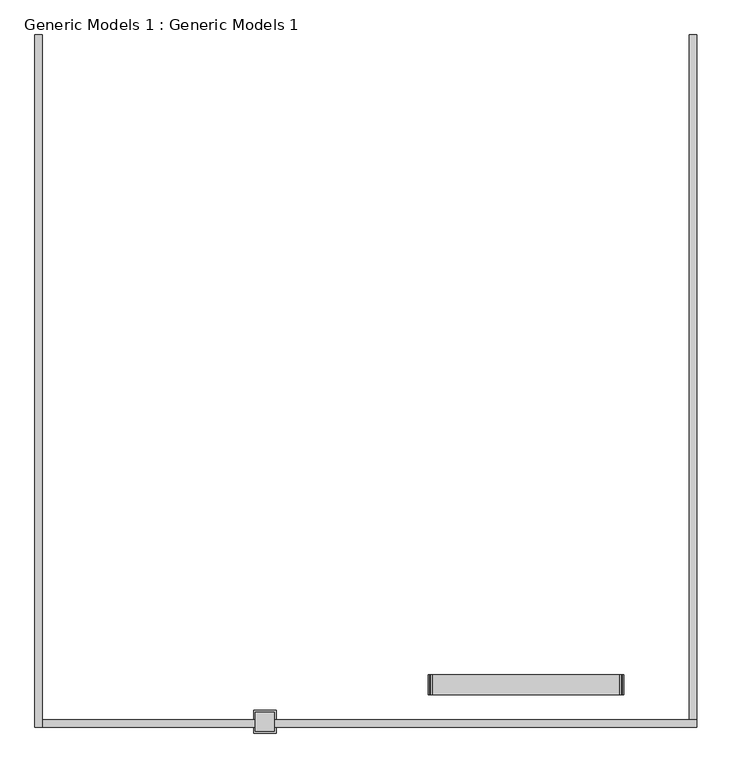
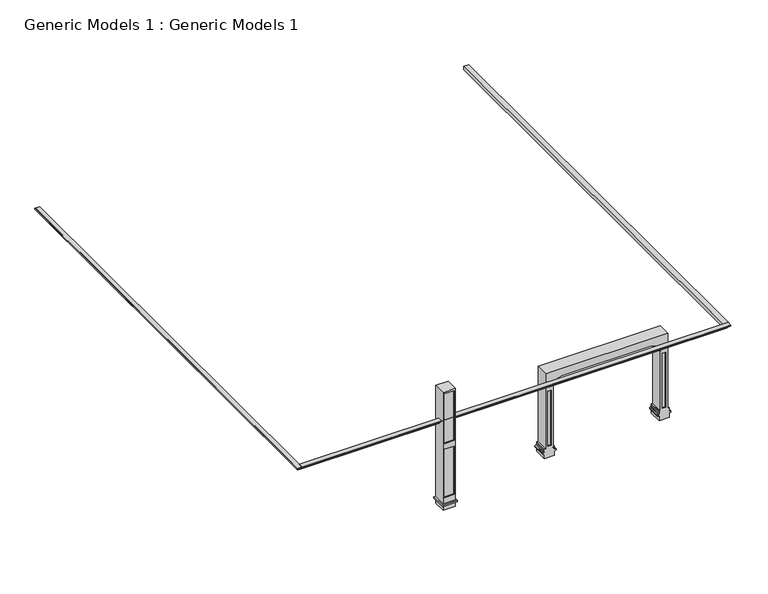
"""IFC4 building model written with IfcOpenShell, lengths in millimetres: proxy geometry, Generic Models 1 : Generic Models 1."""

from ifc_helpers import new_model, si_unit, point, frame, frame_2d, origin, origin_with_axes, place, context, project, spatial, polyline, circle_curve, ellipse_curve, trimmed, segment, composite_curve, outline, extrude, faceted_brep, source, transform, mapped, element, save
from ifc_brep_helpers import plane_surface, cylinder_surface, revolved_surface, advanced_brep


def generic_models_1_generic_models_1_5e55def3(model_context):
    return source(origin(), model_context, "Body", "SolidModel", [
        faceted_brep([(-2619.8591656, -8802.2949916, 5105.4), (-3127.8591656, -8802.2949916, 5105.4), (-3127.8591656, -9310.2949916, 5105.4), (-2619.8591656, -9310.2949916, 5105.4), (-2619.8591656, -8802.2949916, 279.4), (-2619.8591656, -9310.2949916, 279.4), (-3127.8591656, -9310.2949916, 279.4), (-3127.8591656, -8802.2949916, 279.4), (-2670.6591656, -9310.2949916, 532.3431413), (-3077.0591656, -9310.2949916, 532.3431413), (-3077.0591656, -9310.2949916, 2624.1375), (-2670.6591656, -9310.2949916, 2624.1375), (-2670.6591656, -9310.2949916, 5029.2), (-2670.6591656, -9310.2949916, 2870.2), (-3077.0591656, -9310.2949916, 2870.2), (-3077.0591656, -9310.2949916, 5029.2), (-2670.6591656, -9259.4949916, 532.3431413), (-2670.6591656, -9259.4949916, 2624.1375), (-3077.0591656, -9259.4949916, 2624.1375), (-3077.0591656, -9259.4949916, 532.3431413), (-2670.6591656, -9259.4949916, 5029.2), (-3077.0591656, -9259.4949916, 5029.2), (-3077.0591656, -9259.4949916, 2870.2), (-2670.6591656, -9259.4949916, 2870.2)], [[[0, 1, 2, 3]], [[4, 5, 6, 7]], [[1, 0, 4, 7]], [[2, 1, 7, 6]], [[3, 2, 6, 5], [8, 9, 10, 11], [12, 13, 14, 15]], [[0, 3, 5, 4]], [[16, 17, 18, 19]], [[20, 21, 22, 23]], [[16, 19, 9, 8]], [[19, 18, 10, 9]], [[18, 17, 11, 10]], [[17, 16, 8, 11]], [[20, 23, 13, 12]], [[23, 22, 14, 13]], [[22, 21, 15, 14]], [[21, 20, 12, 15]]]),
        extrude(outline(polyline([(-3178.6591656, -9361.0949916), (-3178.6591656, -8751.4949916), (-2569.0591656, -8751.4949916), (-2569.0591656, -9361.0949916), (-3178.6591656, -9361.0949916)])), frame((0.0, 0.0, 203.2), z_axis=(0.0, 0.0, 1.0), x_axis=(1.0, 0.0, 0.0)), (0.0, 0.0, 1.0), 76.2),
        extrude(outline(polyline([(-3127.8591656, -9310.2949916), (-3127.8591656, -8802.2949916), (-2619.8591656, -8802.2949916), (-2619.8591656, -9310.2949916), (-3127.8591656, -9310.2949916)])), origin_with_axes(), (0.0, 0.0, 1.0), 203.2),
        advanced_brep(
        [(-9051.9249265, 9396.8050084, 3810.0), (-8848.7249265, 9396.8050084, 3810.0), (-8848.7249265, 9396.8050084, 3657.6), (-8924.9249265, 9396.8050084, 3657.6), (-8924.9249265, 9396.8050084, 3668.8560823), (-8939.0688442, 9396.8050084, 3683.0), (-8950.3249265, 9396.8050084, 3683.0), (-8950.3249265, 9396.8050084, 3708.4), (-8975.7249265, 9396.8050084, 3733.8), (-9001.1249265, 9396.8050084, 3733.8), (-9001.1249265, 9396.8050084, 3761.8750168), (-9023.8499097, 9396.8050084, 3784.6), (-9026.5249265, 9396.8050084, 3784.6), (-9051.9249265, 9396.8050084, 3784.6), (-9051.9249265, -9180.6199748, 3784.6), (-9051.9249265, -9183.2949916, 3784.6), (-9051.9249265, -9208.6949916, 3784.6), (-9051.9249265, -9208.6949916, 3810.0), (-9026.5249265, -9180.6199748, 3784.6), (-9026.5249265, -9183.2949916, 3784.6), (-9026.5249265, -9208.6949916, 3784.6), (-9023.8499097, -9180.6199748, 3784.6), (-8848.7249265, -9180.6199748, 3784.6), (-8848.7249265, -9208.6949916, 3784.6), (-9001.1249265, -9157.8949916, 3761.8750168), (-9001.1249265, -9157.8949916, 3733.8), (-8975.7249265, -9132.4949916, 3733.8), (-8848.7249265, -9132.4949916, 3733.8), (-8848.7249265, -9157.8949916, 3733.8), (-8950.3249265, -9107.0949916, 3708.4), (-8950.3249265, -9107.0949916, 3683.0), (-8939.0688442, -9095.8389093, 3683.0), (-8848.7249265, -9095.8389093, 3683.0), (-8848.7249265, -9107.0949916, 3683.0), (-8924.9249265, -9081.6949916, 3668.8560823), (-8924.9249265, -9081.6949916, 3657.6), (-8848.7249265, -9081.6949916, 3657.6), (-8848.7249265, -9208.6949916, 3810.0), (-8848.7249265, -9157.8949916, 3761.8750168), (-8848.7249265, -9107.0949916, 3708.4), (-8848.7249265, -9081.6949916, 3668.8560823)],
        [
            (0, 1),
            (1, 2),
            (2, 3),
            (3, 4),
            (4, 5, circle_curve(frame((-8939.0688442, 9396.8050084, 3668.8560823), z_axis=(0.0, -1.0, 0.0), x_axis=(0.0, 0.0, 1.0)), 14.1439177)),
            (5, 6),
            (6, 7),
            (7, 8, circle_curve(frame((-8975.7249265, 9396.8050084, 3708.4), z_axis=(0.0, -1.0, 0.0), x_axis=(0.0, 0.0, 1.0)), 25.4)),
            (8, 9),
            (9, 10),
            (10, 11, circle_curve(frame((-9023.8499097, 9396.8050084, 3761.8750168), z_axis=(0.0, -1.0, 0.0), x_axis=(0.0, 0.0, 1.0)), 22.7249832)),
            (11, 12),
            (12, 13),
            (13, 0),
            (13, 14),
            (14, 15),
            (15, 16),
            (16, 17),
            (17, 0),
            (12, 18),
            (18, 19),
            (19, 20),
            (20, 16),
            (11, 21),
            (21, 22),
            (22, 23),
            (23, 20),
            (10, 24),
            (24, 21, ellipse_curve(frame((-9023.8499097, -9180.6199748, 3761.8750168), z_axis=(0.7071067811865451, -0.7071067811865498, 0.0), x_axis=(-0.7071067811865497, -0.7071067811865452, 0.0)), 32.1379795, 22.7249832)),
            (9, 25),
            (25, 24),
            (8, 26),
            (26, 27),
            (27, 28),
            (28, 25),
            (7, 29),
            (29, 26, ellipse_curve(frame((-8975.7249265, -9132.4949916, 3708.4), z_axis=(0.7071067811865451, -0.7071067811865498, 0.0), x_axis=(-0.7071067811865497, -0.7071067811865452, 0.0)), 35.9210245, 25.4)),
            (6, 30),
            (30, 29),
            (5, 31),
            (31, 32),
            (32, 33),
            (33, 30),
            (4, 34),
            (34, 31, ellipse_curve(frame((-8939.0688442, -9095.8389093, 3668.8560823), z_axis=(0.7071067811865451, -0.7071067811865498, 0.0), x_axis=(-0.7071067811865497, -0.7071067811865452, 0.0)), 20.0025203, 14.1439177)),
            (3, 35),
            (35, 34),
            (2, 36),
            (36, 35),
            (1, 37),
            (37, 23),
            (22, 38, circle_curve(frame((-8848.7249265, -9180.6199748, 3761.8750168), z_axis=(-1.0, 0.0, 0.0), x_axis=(0.0, 0.0, 1.0)), 22.7249832)),
            (38, 28),
            (27, 39, circle_curve(frame((-8848.7249265, -9132.4949916, 3708.4), z_axis=(-1.0, 0.0, 0.0), x_axis=(0.0, 0.0, 1.0)), 25.4)),
            (39, 33),
            (32, 40, circle_curve(frame((-8848.7249265, -9095.8389093, 3668.8560823), z_axis=(-1.0, 0.0, 0.0), x_axis=(0.0, 0.0, 1.0)), 14.1439177)),
            (40, 36),
            (17, 37),
            (40, 34),
            (24, 38),
            (29, 39),
        ],
        [
            plane_surface(frame((-8848.7249265, 9396.8050084, 3810.0), z_axis=(0.0, 1.0, 0.0), x_axis=(1.0, 0.0, 0.0))),
            plane_surface(frame((-9051.9249265, 9396.8050084, 3784.6), z_axis=(-1.0, 0.0, 0.0), x_axis=(0.0, -1.0, 0.0))),
            plane_surface(frame((-9026.5249265, 9396.8050084, 3784.6), z_axis=(0.0, 0.0, -1.0), x_axis=(0.0, -1.0, 0.0))),
            plane_surface(frame((-9023.8499097, 9396.8050084, 3784.6), z_axis=(0.0, 0.0, -1.0), x_axis=(0.0, -1.0, 0.0))),
            revolved_surface(polyline([(-9023.8499097, -9203.344958038084, 3784.6000000000004), (-9023.8499097, 9396.8050084, 3784.6000000000004)]), (-9023.8499097, -9241.2899429, 3761.8750168), (0.0, -1.0, 0.0)),
            plane_surface(frame((-9001.1249265, 9396.8050084, 3733.8), z_axis=(-1.0, 0.0, 0.0), x_axis=(0.0, -1.0, 0.0))),
            plane_surface(frame((-8975.7249265, 9396.8050084, 3733.8), z_axis=(0.0, 0.0, -1.0), x_axis=(0.0, -1.0, 0.0))),
            revolved_surface(polyline([(-8975.7249265, -9157.894991611118, 3733.8), (-8975.7249265, 9396.8050084, 3733.8)]), (-8975.7249265, -9241.2899429, 3708.4), (0.0, -1.0, 0.0)),
            plane_surface(frame((-8950.3249265, 9396.8050084, 3683.0), z_axis=(-1.0, 0.0, 0.0), x_axis=(0.0, -1.0, 0.0))),
            plane_surface(frame((-8939.0688442, 9396.8050084, 3683.0), z_axis=(0.0, 0.0, -1.0), x_axis=(0.0, -1.0, 0.0))),
            revolved_surface(polyline([(-8939.0688442, -9109.982827044953, 3683.0), (-8939.0688442, 9396.8050084, 3683.0)]), (-8939.0688442, -9241.2899429, 3668.8560823), (0.0, -1.0, 0.0)),
            plane_surface(frame((-8924.9249265, 9396.8050084, 3657.6), z_axis=(-1.0, 0.0, 0.0), x_axis=(0.0, -1.0, 0.0))),
            plane_surface(frame((-8848.7249265, 9396.8050084, 3657.6), z_axis=(0.0, 0.0, -1.0), x_axis=(0.0, -1.0, 0.0))),
            plane_surface(frame((-8848.7249265, 9396.8050084, 3810.0), z_axis=(1.0, 0.0, 0.0), x_axis=(0.0, -1.0, 0.0))),
            plane_surface(frame((-9051.9249265, 9396.8050084, 3810.0), z_axis=(0.0, 0.0, 1.0), x_axis=(0.0, -1.0, 0.0))),
            plane_surface(frame((-9178.6298394, -9081.6949916, 3668.8560823), z_axis=(0.0, -1.0, 0.0), x_axis=(1.0, 0.0, 0.0))),
            plane_surface(frame((-9178.6298394, -9208.6949916, 3810.0), z_axis=(0.0, -1.0, 0.0), x_axis=(1.0, 0.0, 0.0))),
            revolved_surface(polyline([(-9046.574892938084, -9180.6199748, 3784.6000000000004), (-8848.7249265, -9180.6199748, 3784.6000000000004)]), (-8848.7249265, -9180.6199748, 3761.8750168), (-1.0, 0.0, 0.0)),
            plane_surface(frame((-9178.6298394, -9157.8949916, 3761.8750168), z_axis=(0.0, -1.0, 0.0), x_axis=(1.0, 0.0, 0.0))),
            revolved_surface(polyline([(-9001.124926511116, -9132.4949916, 3733.8), (-8848.7249265, -9132.4949916, 3733.8)]), (-8848.7249265, -9132.4949916, 3708.4), (-1.0, 0.0, 0.0)),
            plane_surface(frame((-9178.6298394, -9107.0949916, 3708.4), z_axis=(0.0, -1.0, 0.0), x_axis=(1.0, 0.0, 0.0))),
            revolved_surface(polyline([(-8953.212761944951, -9095.8389093, 3683.0), (-8848.7249265, -9095.8389093, 3683.0)]), (-8848.7249265, -9095.8389093, 3668.8560823), (-1.0, 0.0, 0.0)),
        ],
        [
            (0, [[1, 2, 3, 4, 5, 6, 7, 8, 9, 10, 11, 12, 13, 14]]),
            (1, [[-14, 15, 16, 17, 18, 19]]),
            (2, [[-13, 20, 21, 22, 23, -17, -16, -15]]),
            (3, [[-12, 24, 25, 26, 27, -22, -21, -20]]),
            (4, [[-11, 28, 29, -24]]),
            (5, [[-10, 30, 31, -28]]),
            (6, [[-9, 32, 33, 34, 35, -30]]),
            (7, [[-8, 36, 37, -32]]),
            (8, [[-7, 38, 39, -36]]),
            (9, [[-6, 40, 41, 42, 43, -38]]),
            (10, [[-5, 44, 45, -40]]),
            (11, [[-4, 46, 47, -44]]),
            (12, [[-3, 48, 49, -46]]),
            (13, [[-2, 50, 51, -26, 52, 53, -34, 54, 55, -42, 56, 57, -48]]),
            (14, [[-1, -19, 58, -50]]),
            (15, [[59, -47, -49, -57]]),
            (16, [[-27, -51, -58, -18, -23]]),
            (17, [[-25, -29, 60, -52]]),
            (18, [[-60, -31, -35, -53]]),
            (19, [[-33, -37, 61, -54]]),
            (20, [[-61, -39, -43, -55]]),
            (21, [[-41, -45, -59, -56]]),
        ],
    ),
        advanced_brep(
        [(8728.0750735, -9208.6949916, 3810.0), (8728.0750735, -9208.6949916, 3784.6), (8728.0750735, -9183.2949916, 3784.6), (8728.0750735, -9005.4949916, 3784.6), (8728.0750735, -9005.4949916, 3810.0), (-8848.7249265, -9208.6949916, 3810.0), (-8848.7249265, -9005.4949916, 3810.0), (-8848.7249265, -9005.4949916, 3657.6), (-8848.7249265, -9081.6949916, 3657.6), (-8848.7249265, -9081.6949916, 3668.8560823), (-8848.7249265, -9095.8389093, 3683.0), (-8848.7249265, -9107.0949916, 3683.0), (-8848.7249265, -9107.0949916, 3708.4), (-8848.7249265, -9132.4949916, 3733.8), (-8848.7249265, -9157.8949916, 3733.8), (-8848.7249265, -9157.8949916, 3761.8750168), (-8848.7249265, -9180.6199748, 3784.6), (-8848.7249265, -9183.2949916, 3784.6), (-8848.7249265, -9208.6949916, 3784.6), (8700.0000567, -9208.6949916, 3784.6), (8700.0000567, -9183.2949916, 3784.6), (8700.0000567, -9180.6199748, 3784.6), (8700.0000567, -9005.4949916, 3784.6), (8677.2750735, -9157.8949916, 3761.8750168), (8677.2750735, -9157.8949916, 3733.8), (8651.8750735, -9132.4949916, 3733.8), (8651.8750735, -9005.4949916, 3733.8), (8677.2750735, -9005.4949916, 3733.8), (8626.4750735, -9107.0949916, 3708.4), (8626.4750735, -9107.0949916, 3683.0), (8615.2189912, -9095.8389093, 3683.0), (8615.2189912, -9005.4949916, 3683.0), (8626.4750735, -9005.4949916, 3683.0), (8601.0750735, -9081.6949916, 3668.8560823), (8601.0750735, -9081.6949916, 3657.6), (8601.0750735, -9005.4949916, 3657.6), (8677.2750735, -9005.4949916, 3761.8750168), (8626.4750735, -9005.4949916, 3708.4), (8601.0750735, -9005.4949916, 3668.8560823)],
        [
            (0, 1),
            (1, 2),
            (2, 3),
            (3, 4),
            (4, 0),
            (5, 6),
            (6, 7),
            (7, 8),
            (8, 9),
            (9, 10, circle_curve(frame((-8848.7249265, -9095.8389093, 3668.8560823), z_axis=(1.0, 0.0, 0.0), x_axis=(0.0, 0.0, 1.0)), 14.1439177)),
            (10, 11),
            (11, 12),
            (12, 13, circle_curve(frame((-8848.7249265, -9132.4949916, 3708.4), z_axis=(1.0, 0.0, 0.0), x_axis=(0.0, 0.0, 1.0)), 25.4)),
            (13, 14),
            (14, 15),
            (15, 16, circle_curve(frame((-8848.7249265, -9180.6199748, 3761.8750168), z_axis=(1.0, 0.0, 0.0), x_axis=(0.0, 0.0, 1.0)), 22.7249832)),
            (16, 17),
            (17, 18),
            (18, 5),
            (0, 5),
            (18, 19),
            (19, 1),
            (17, 20),
            (20, 2),
            (16, 21),
            (21, 22),
            (22, 3),
            (15, 23),
            (23, 21, ellipse_curve(frame((8700.0000567, -9180.6199748, 3761.8750168), z_axis=(0.7071067811865475, 0.7071067811865475, 0.0), x_axis=(-0.7071067811865476, 0.7071067811865474, 0.0)), 32.1379795, 22.7249832)),
            (14, 24),
            (24, 23),
            (13, 25),
            (25, 26),
            (26, 27),
            (27, 24),
            (12, 28),
            (28, 25, ellipse_curve(frame((8651.8750735, -9132.4949916, 3708.4), z_axis=(0.7071067811865475, 0.7071067811865475, 0.0), x_axis=(-0.7071067811865476, 0.7071067811865474, 0.0)), 35.9210245, 25.4)),
            (11, 29),
            (29, 28),
            (10, 30),
            (30, 31),
            (31, 32),
            (32, 29),
            (9, 33),
            (33, 30, ellipse_curve(frame((8615.2189912, -9095.8389093, 3668.8560823), z_axis=(0.7071067811865475, 0.7071067811865475, 0.0), x_axis=(-0.7071067811865476, 0.7071067811865474, 0.0)), 20.0025203, 14.1439177)),
            (8, 34),
            (34, 33),
            (7, 35),
            (35, 34),
            (6, 4),
            (22, 36, circle_curve(frame((8700.0000567, -9005.4949916, 3761.8750168), z_axis=(0.0, -1.0, 0.0), x_axis=(0.0, 0.0, 1.0)), 22.7249832)),
            (36, 27),
            (26, 37, circle_curve(frame((8651.8750735, -9005.4949916, 3708.4), z_axis=(0.0, -1.0, 0.0), x_axis=(0.0, 0.0, 1.0)), 25.4)),
            (37, 32),
            (31, 38, circle_curve(frame((8615.2189912, -9005.4949916, 3668.8560823), z_axis=(0.0, -1.0, 0.0), x_axis=(0.0, 0.0, 1.0)), 14.1439177)),
            (38, 35),
            (36, 23),
            (28, 37),
            (33, 38),
        ],
        [
            plane_surface(frame((8728.0750735, -9208.6949916, 3810.0), z_axis=(1.0, 0.0, 0.0), x_axis=(0.0, 0.0, -1.0))),
            plane_surface(frame((-8848.7249265, -9208.6949916, 3810.0), z_axis=(-1.0, 0.0, 0.0), x_axis=(0.0, 0.0, 1.0))),
            plane_surface(frame((8728.0750735, -9208.6949916, 3810.0), z_axis=(0.0, -1.0, 0.0), x_axis=(-1.0, 0.0, 0.0))),
            plane_surface(frame((8728.0750735, -9208.6949916, 3784.6), z_axis=(0.0, 0.0, -1.0), x_axis=(-1.0, 0.0, 0.0))),
            plane_surface(frame((8728.0750735, -9183.2949916, 3784.6), z_axis=(0.0, 0.0, -1.0), x_axis=(-1.0, 0.0, 0.0))),
            revolved_surface(polyline([(-8848.7249265, -9180.6199748, 3784.6000000000004), (8722.725039938086, -9180.6199748, 3784.6000000000004)]), (-8848.7249265, -9180.6199748, 3761.8750168), (-1.0, 0.0, 0.0)),
            plane_surface(frame((8728.0750735, -9157.8949916, 3761.8750168), z_axis=(0.0, -1.0, 0.0), x_axis=(-1.0, 0.0, 0.0))),
            plane_surface(frame((8728.0750735, -9157.8949916, 3733.8), z_axis=(0.0, 0.0, -1.0), x_axis=(-1.0, 0.0, 0.0))),
            revolved_surface(polyline([(-8848.7249265, -9132.4949916, 3733.8), (8677.275073511119, -9132.4949916, 3733.8)]), (-8848.7249265, -9132.4949916, 3708.4), (-1.0, 0.0, 0.0)),
            plane_surface(frame((8728.0750735, -9107.0949916, 3708.4), z_axis=(0.0, -1.0, 0.0), x_axis=(-1.0, 0.0, 0.0))),
            plane_surface(frame((8728.0750735, -9107.0949916, 3683.0), z_axis=(0.0, 0.0, -1.0), x_axis=(-1.0, 0.0, 0.0))),
            revolved_surface(polyline([(-8848.7249265, -9095.8389093, 3683.0), (8629.36290894495, -9095.8389093, 3683.0)]), (-8848.7249265, -9095.8389093, 3668.8560823), (-1.0, 0.0, 0.0)),
            plane_surface(frame((8728.0750735, -9081.6949916, 3668.8560823), z_axis=(0.0, -1.0, 0.0), x_axis=(-1.0, 0.0, 0.0))),
            plane_surface(frame((8728.0750735, -9081.6949916, 3657.6), z_axis=(0.0, 0.0, -1.0), x_axis=(-1.0, 0.0, 0.0))),
            plane_surface(frame((8728.0750735, -9005.4949916, 3657.6), z_axis=(0.0, 1.0, 0.0), x_axis=(-1.0, 0.0, 0.0))),
            plane_surface(frame((8728.0750735, -9005.4949916, 3810.0), z_axis=(0.0, 0.0, 1.0), x_axis=(-1.0, 0.0, 0.0))),
            plane_surface(frame((8677.2750735, -9313.9893906, 3761.8750168), z_axis=(1.0, 0.0, 0.0), x_axis=(0.0, 1.0, 0.0))),
            revolved_surface(polyline([(8651.8750735, -9157.894991611118, 3733.8), (8651.8750735, -9005.4949916, 3733.8)]), (8651.8750735, -9005.4949916, 3708.4), (0.0, -1.0, 0.0)),
            plane_surface(frame((8626.4750735, -9313.9893906, 3708.4), z_axis=(1.0, 0.0, 0.0), x_axis=(0.0, 1.0, 0.0))),
            revolved_surface(polyline([(8615.2189912, -9109.982827044953, 3683.0), (8615.2189912, -9005.4949916, 3683.0)]), (8615.2189912, -9005.4949916, 3668.8560823), (0.0, -1.0, 0.0)),
            plane_surface(frame((8601.0750735, -9313.9893906, 3668.8560823), z_axis=(1.0, 0.0, 0.0), x_axis=(0.0, 1.0, 0.0))),
            revolved_surface(polyline([(8700.0000567, -9203.344958038084, 3784.6000000000004), (8700.0000567, -9005.4949916, 3784.6000000000004)]), (8700.0000567, -9005.4949916, 3761.8750168), (0.0, -1.0, 0.0)),
        ],
        [
            (0, [[1, 2, 3, 4, 5]]),
            (1, [[6, 7, 8, 9, 10, 11, 12, 13, 14, 15, 16, 17, 18, 19]]),
            (2, [[-1, 20, -19, 21, 22]]),
            (3, [[-2, -22, -21, -18, 23, 24]]),
            (4, [[-24, -23, -17, 25, 26, 27, -3]]),
            (5, [[-16, 28, 29, -25]]),
            (6, [[-15, 30, 31, -28]]),
            (7, [[-14, 32, 33, 34, 35, -30]]),
            (8, [[-13, 36, 37, -32]]),
            (9, [[-12, 38, 39, -36]]),
            (10, [[-11, 40, 41, 42, 43, -38]]),
            (11, [[-10, 44, 45, -40]]),
            (12, [[-9, 46, 47, -44]]),
            (13, [[-8, 48, 49, -46]]),
            (14, [[-7, 50, -4, -27, 51, 52, -34, 53, 54, -42, 55, 56, -48]]),
            (15, [[-5, -50, -6, -20]]),
            (16, [[57, -31, -35, -52]]),
            (17, [[-33, -37, 58, -53]]),
            (18, [[-58, -39, -43, -54]]),
            (19, [[-41, -45, 59, -55]]),
            (20, [[-59, -47, -49, -56]]),
            (21, [[-26, -29, -57, -51]]),
        ],
    ),
        extrude(outline(composite_curve([segment(polyline([(3810.0, 8728.0750735), (3810.0, 8524.8750735), (3657.6, 8524.8750735), (3657.6, 8601.0750735), (3668.8560823, 8601.0750735)]), True, "CONTINUOUS"), segment(trimmed(circle_curve(frame_2d((3668.8560823, 8615.2189912)), 14.1439177), [point((3668.8560823, 8601.0750735))], [point((3683.0, 8615.2189912))], True, "CARTESIAN"), True, "CONTINUOUS"), segment(polyline([(3683.0, 8615.2189912), (3683.0, 8626.4750735), (3708.4, 8626.4750735)]), True, "CONTINUOUS"), segment(trimmed(circle_curve(frame_2d((3708.4, 8651.8750735)), 25.4), [point((3708.4, 8626.4750735))], [point((3733.8, 8651.8750735))], True, "CARTESIAN"), True, "CONTINUOUS"), segment(polyline([(3733.8, 8651.8750735), (3733.8, 8677.2750735), (3761.8750168, 8677.2750735)]), True, "CONTINUOUS"), segment(trimmed(circle_curve(frame_2d((3761.8750168, 8700.0000567)), 22.7249832), [point((3761.8750168, 8677.2750735))], [point((3784.6, 8700.0000567))], True, "CARTESIAN"), True, "CONTINUOUS"), segment(polyline([(3784.6, 8700.0000567), (3784.6, 8702.6750735), (3784.6, 8728.0750735), (3810.0, 8728.0750735)]), True, "CONTINUOUS")], self_intersect=False)), frame((0.0, -9005.4949916, 0.0), z_axis=(0.0, 1.0, 0.0), x_axis=(0.0, 0.0, 1.0)), (0.0, 0.0, 1.0), 18402.3),
        advanced_brep(
        [(6645.2750735, -7793.5697181, 3657.6), (6645.2750735, -7793.5697181, 406.4), (6696.0750735, -7793.5697181, 406.4), (6696.0750735, -7793.5697181, 355.6), (6696.0750735, -7793.5697181, 304.8), (6721.4750735, -7793.5697181, 279.4), (6740.5250735, -7793.5697181, 279.4), (6772.2750735, -7793.5697181, 247.65), (6772.2750735, -7793.5697181, 228.6), (6746.8750735, -7793.5697181, 203.2), (6717.4871849, -7793.5697181, 203.2), (6696.0750735, -7793.5697181, 181.7878886), (6696.0750735, -7793.5697181, 0.0), (6289.6750735, -7793.5697181, 0.0), (6289.6750735, -7793.5697181, 181.7878886), (6268.2629621, -7793.5697181, 203.2), (6238.8750735, -7793.5697181, 203.2), (6213.4750735, -7793.5697181, 228.6), (6213.4750735, -7793.5697181, 247.65), (6245.2250735, -7793.5697181, 279.4), (6264.2750735, -7793.5697181, 279.4), (6289.6750735, -7793.5697181, 304.8), (6289.6750735, -7793.5697181, 355.6), (6289.6750735, -7793.5697181, 406.4), (6340.4750735, -7793.5697181, 406.4), (6340.4750735, -7793.5697181, 2946.4), (5934.0750735, -7793.5697181, 3352.8), (2351.7254689, -7793.5697181, 3352.8), (1945.3254689, -7793.5697181, 2946.4), (1945.3254689, -7793.5697181, 406.4), (1996.1254689, -7793.5697181, 406.4), (1996.1254689, -7793.5697181, 355.6), (1996.1254689, -7793.5697181, 304.8), (2021.5254689, -7793.5697181, 279.4), (2040.5754689, -7793.5697181, 279.4), (2072.3254689, -7793.5697181, 247.65), (2072.3254689, -7793.5697181, 228.6), (2046.9254689, -7793.5697181, 203.2), (2017.5375803, -7793.5697181, 203.2), (1996.1254689, -7793.5697181, 181.7878886), (1996.1254689, -7793.5697181, 0.0), (1589.7254689, -7793.5697181, 0.0), (1589.7254689, -7793.5697181, 181.7878886), (1568.3133575, -7793.5697181, 203.2), (1538.9254689, -7793.5697181, 203.2), (1513.5254689, -7793.5697181, 228.6), (1513.5254689, -7793.5697181, 247.65), (1545.2754689, -7793.5697181, 279.4), (1564.3254689, -7793.5697181, 279.4), (1589.7254689, -7793.5697181, 304.8), (1589.7254689, -7793.5697181, 355.6), (1589.7254689, -7793.5697181, 406.4), (1640.5254689, -7793.5697181, 406.4), (1640.5254689, -7793.5697181, 3657.6), (6645.2750735, -8332.8472664, 3657.6), (1640.5254689, -8332.8472664, 3657.6), (1640.5254689, -8332.8472664, 406.4), (1589.7254689, -8332.8472664, 406.4), (1589.7254689, -8332.8472664, 355.6), (1589.7254689, -8332.8472664, 304.8), (1564.3254689, -8332.8472664, 279.4), (1545.2754689, -8332.8472664, 279.4), (1513.5254689, -8332.8472664, 247.65), (1513.5254689, -8332.8472664, 228.6), (1538.9254689, -8332.8472664, 203.2), (1568.3133575, -8332.8472664, 203.2), (1589.7254689, -8332.8472664, 181.7878886), (1589.7254689, -8332.8472664, 0.0), (1996.1254689, -8332.8472664, 0.0), (1996.1254689, -8332.8472664, 181.7878886), (2017.5375803, -8332.8472664, 203.2), (2046.9254689, -8332.8472664, 203.2), (2072.3254689, -8332.8472664, 228.6), (2072.3254689, -8332.8472664, 247.65), (2040.5754689, -8332.8472664, 279.4), (2021.5254689, -8332.8472664, 279.4), (1996.1254689, -8332.8472664, 304.8), (1996.1254689, -8332.8472664, 355.6), (1996.1254689, -8332.8472664, 406.4), (1945.3254689, -8332.8472664, 406.4), (1945.3254689, -8332.8472664, 2946.4), (2351.7254689, -8332.8472664, 3352.8), (5934.0750735, -8332.8472664, 3352.8), (6340.4750735, -8332.8472664, 2946.4), (6340.4750735, -8332.8472664, 406.4), (6289.6750735, -8332.8472664, 406.4), (6289.6750735, -8332.8472664, 355.6), (6289.6750735, -8332.8472664, 304.8), (6264.2750735, -8332.8472664, 279.4), (6245.2250735, -8332.8472664, 279.4), (6213.4750735, -8332.8472664, 247.65), (6213.4750735, -8332.8472664, 228.6), (6238.8750735, -8332.8472664, 203.2), (6268.2629621, -8332.8472664, 203.2), (6289.6750735, -8332.8472664, 181.7878886), (6289.6750735, -8332.8472664, 0.0), (6696.0750735, -8332.8472664, 0.0), (6696.0750735, -8332.8472664, 181.7878886), (6717.4871849, -8332.8472664, 203.2), (6746.8750735, -8332.8472664, 203.2), (6772.2750735, -8332.8472664, 228.6), (6772.2750735, -8332.8472664, 247.65), (6740.5250735, -8332.8472664, 279.4), (6721.4750735, -8332.8472664, 279.4), (6696.0750735, -8332.8472664, 304.8), (6696.0750735, -8332.8472664, 355.6), (6696.0750735, -8332.8472664, 406.4), (6645.2750735, -8332.8472664, 406.4), (1869.1254689, -8332.8472664, 482.6), (1716.7254689, -8332.8472664, 482.6), (1716.7254689, -8332.8472664, 2870.2), (1869.1254689, -8332.8472664, 2870.2), (6569.0750735, -8332.8472664, 482.6), (6416.6750735, -8332.8472664, 482.6), (6416.6750735, -8332.8472664, 2870.2), (6569.0750735, -8332.8472664, 2870.2), (1869.1254689, -8282.0472664, 482.6), (1869.1254689, -8282.0472664, 2870.2), (1716.7254689, -8282.0472664, 2870.2), (1716.7254689, -8282.0472664, 482.6), (6569.0750735, -8282.0472664, 482.6), (6569.0750735, -8282.0472664, 2870.2), (6416.6750735, -8282.0472664, 2870.2), (6416.6750735, -8282.0472664, 482.6)],
        [
            (0, 1),
            (1, 2),
            (2, 3),
            (3, 4),
            (4, 5, circle_curve(frame((6721.4750735, -7793.5697181, 304.8), z_axis=(0.0, -1.0, 0.0), x_axis=(1.0, 0.0, 0.0)), 25.4)),
            (5, 6),
            (6, 7, circle_curve(frame((6740.5250735, -7793.5697181, 247.65), z_axis=(0.0, 1.0, 0.0), x_axis=(1.0, 0.0, 0.0)), 31.75)),
            (7, 8),
            (8, 9, circle_curve(frame((6746.8750735, -7793.5697181, 228.6), z_axis=(0.0, 1.0, 0.0), x_axis=(1.0, 0.0, 0.0)), 25.4)),
            (9, 10),
            (10, 11, circle_curve(frame((6717.4871849, -7793.5697181, 181.7878886), z_axis=(0.0, -1.0, 0.0), x_axis=(1.0, 0.0, 0.0)), 21.4121114)),
            (11, 12),
            (12, 13),
            (13, 14),
            (14, 15, circle_curve(frame((6268.2629621, -7793.5697181, 181.7878886), z_axis=(0.0, -1.0, 0.0), x_axis=(-1.0, 0.0, 0.0)), 21.4121114)),
            (15, 16),
            (16, 17, circle_curve(frame((6238.8750735, -7793.5697181, 228.6), z_axis=(0.0, 1.0, 0.0), x_axis=(-1.0, 0.0, 0.0)), 25.4)),
            (17, 18),
            (18, 19, circle_curve(frame((6245.2250735, -7793.5697181, 247.65), z_axis=(0.0, 1.0, 0.0), x_axis=(-1.0, 0.0, 0.0)), 31.75)),
            (19, 20),
            (20, 21, circle_curve(frame((6264.2750735, -7793.5697181, 304.8), z_axis=(0.0, -1.0, 0.0), x_axis=(-1.0, 0.0, 0.0)), 25.4)),
            (21, 22),
            (22, 23),
            (23, 24),
            (24, 25),
            (25, 26, circle_curve(frame((5934.0750735, -7793.5697181, 2946.4), z_axis=(0.0, -1.0, 0.0), x_axis=(-1.0, 0.0, 0.0)), 406.4)),
            (26, 27),
            (27, 28, circle_curve(frame((2351.7254689, -7793.5697181, 2946.4), z_axis=(0.0, -1.0, 0.0), x_axis=(-1.0, 0.0, 0.0)), 406.4)),
            (28, 29),
            (29, 30),
            (30, 31),
            (31, 32),
            (32, 33, circle_curve(frame((2021.5254689, -7793.5697181, 304.8), z_axis=(0.0, -1.0, 0.0), x_axis=(1.0, 0.0, 0.0)), 25.4)),
            (33, 34),
            (34, 35, circle_curve(frame((2040.5754689, -7793.5697181, 247.65), z_axis=(0.0, 1.0, 0.0), x_axis=(1.0, 0.0, 0.0)), 31.75)),
            (35, 36),
            (36, 37, circle_curve(frame((2046.9254689, -7793.5697181, 228.6), z_axis=(0.0, 1.0, 0.0), x_axis=(1.0, 0.0, 0.0)), 25.4)),
            (37, 38),
            (38, 39, circle_curve(frame((2017.5375803, -7793.5697181, 181.7878886), z_axis=(0.0, -1.0, 0.0), x_axis=(1.0, 0.0, 0.0)), 21.4121114)),
            (39, 40),
            (40, 41),
            (41, 42),
            (42, 43, circle_curve(frame((1568.3133575, -7793.5697181, 181.7878886), z_axis=(0.0, -1.0, 0.0), x_axis=(-1.0, 0.0, 0.0)), 21.4121114)),
            (43, 44),
            (44, 45, circle_curve(frame((1538.9254689, -7793.5697181, 228.6), z_axis=(0.0, 1.0, 0.0), x_axis=(-1.0, 0.0, 0.0)), 25.4)),
            (45, 46),
            (46, 47, circle_curve(frame((1545.2754689, -7793.5697181, 247.65), z_axis=(0.0, 1.0, 0.0), x_axis=(-1.0, 0.0, 0.0)), 31.75)),
            (47, 48),
            (48, 49, circle_curve(frame((1564.3254689, -7793.5697181, 304.8), z_axis=(0.0, -1.0, 0.0), x_axis=(-1.0, 0.0, 0.0)), 25.4)),
            (49, 50),
            (50, 51),
            (51, 52),
            (52, 53),
            (53, 0),
            (54, 55),
            (55, 56),
            (56, 57),
            (57, 58),
            (58, 59),
            (59, 60, circle_curve(frame((1564.3254689, -8332.8472664, 304.8), z_axis=(0.0, 1.0, 0.0), x_axis=(-1.0, 0.0, 0.0)), 25.4)),
            (60, 61),
            (61, 62, circle_curve(frame((1545.2754689, -8332.8472664, 247.65), z_axis=(0.0, -1.0, 0.0), x_axis=(-1.0, 0.0, 0.0)), 31.75)),
            (62, 63),
            (63, 64, circle_curve(frame((1538.9254689, -8332.8472664, 228.6), z_axis=(0.0, -1.0, 0.0), x_axis=(-1.0, 0.0, 0.0)), 25.4)),
            (64, 65),
            (65, 66, circle_curve(frame((1568.3133575, -8332.8472664, 181.7878886), z_axis=(0.0, 1.0, 0.0), x_axis=(-1.0, 0.0, 0.0)), 21.4121114)),
            (66, 67),
            (67, 68),
            (68, 69),
            (69, 70, circle_curve(frame((2017.5375803, -8332.8472664, 181.7878886), z_axis=(0.0, 1.0, 0.0), x_axis=(1.0, 0.0, 0.0)), 21.4121114)),
            (70, 71),
            (71, 72, circle_curve(frame((2046.9254689, -8332.8472664, 228.6), z_axis=(0.0, -1.0, 0.0), x_axis=(1.0, 0.0, 0.0)), 25.4)),
            (72, 73),
            (73, 74, circle_curve(frame((2040.5754689, -8332.8472664, 247.65), z_axis=(0.0, -1.0, 0.0), x_axis=(1.0, 0.0, 0.0)), 31.75)),
            (74, 75),
            (75, 76, circle_curve(frame((2021.5254689, -8332.8472664, 304.8), z_axis=(0.0, 1.0, 0.0), x_axis=(1.0, 0.0, 0.0)), 25.4)),
            (76, 77),
            (77, 78),
            (78, 79),
            (79, 80),
            (80, 81, circle_curve(frame((2351.7254689, -8332.8472664, 2946.4), z_axis=(0.0, 1.0, 0.0), x_axis=(-1.0, 0.0, 0.0)), 406.4)),
            (81, 82),
            (82, 83, circle_curve(frame((5934.0750735, -8332.8472664, 2946.4), z_axis=(0.0, 1.0, 0.0), x_axis=(-1.0, 0.0, 0.0)), 406.4)),
            (83, 84),
            (84, 85),
            (85, 86),
            (86, 87),
            (87, 88, circle_curve(frame((6264.2750735, -8332.8472664, 304.8), z_axis=(0.0, 1.0, 0.0), x_axis=(-1.0, 0.0, 0.0)), 25.4)),
            (88, 89),
            (89, 90, circle_curve(frame((6245.2250735, -8332.8472664, 247.65), z_axis=(0.0, -1.0, 0.0), x_axis=(-1.0, 0.0, 0.0)), 31.75)),
            (90, 91),
            (91, 92, circle_curve(frame((6238.8750735, -8332.8472664, 228.6), z_axis=(0.0, -1.0, 0.0), x_axis=(-1.0, 0.0, 0.0)), 25.4)),
            (92, 93),
            (93, 94, circle_curve(frame((6268.2629621, -8332.8472664, 181.7878886), z_axis=(0.0, 1.0, 0.0), x_axis=(-1.0, 0.0, 0.0)), 21.4121114)),
            (94, 95),
            (95, 96),
            (96, 97),
            (97, 98, circle_curve(frame((6717.4871849, -8332.8472664, 181.7878886), z_axis=(0.0, 1.0, 0.0), x_axis=(1.0, 0.0, 0.0)), 21.4121114)),
            (98, 99),
            (99, 100, circle_curve(frame((6746.8750735, -8332.8472664, 228.6), z_axis=(0.0, -1.0, 0.0), x_axis=(1.0, 0.0, 0.0)), 25.4)),
            (100, 101),
            (101, 102, circle_curve(frame((6740.5250735, -8332.8472664, 247.65), z_axis=(0.0, -1.0, 0.0), x_axis=(1.0, 0.0, 0.0)), 31.75)),
            (102, 103),
            (103, 104, circle_curve(frame((6721.4750735, -8332.8472664, 304.8), z_axis=(0.0, 1.0, 0.0), x_axis=(1.0, 0.0, 0.0)), 25.4)),
            (104, 105),
            (105, 106),
            (106, 107),
            (107, 54),
            (108, 109),
            (109, 110),
            (110, 111),
            (111, 108),
            (112, 113),
            (113, 114),
            (114, 115),
            (115, 112),
            (0, 54),
            (107, 1),
            (106, 2),
            (105, 3),
            (104, 4),
            (103, 5),
            (102, 6),
            (101, 7),
            (100, 8),
            (99, 9),
            (98, 10),
            (97, 11),
            (96, 12),
            (95, 13),
            (94, 14),
            (93, 15),
            (92, 16),
            (91, 17),
            (90, 18),
            (89, 19),
            (88, 20),
            (87, 21),
            (86, 22),
            (85, 23),
            (84, 24),
            (83, 25),
            (82, 26),
            (81, 27),
            (80, 28),
            (79, 29),
            (52, 56),
            (55, 53),
            (78, 30),
            (77, 31),
            (76, 32),
            (75, 33),
            (74, 34),
            (73, 35),
            (72, 36),
            (71, 37),
            (70, 38),
            (69, 39),
            (68, 40),
            (67, 41),
            (66, 42),
            (65, 43),
            (64, 44),
            (63, 45),
            (62, 46),
            (61, 47),
            (60, 48),
            (59, 49),
            (58, 50),
            (57, 51),
            (116, 117),
            (117, 118),
            (118, 119),
            (119, 116),
            (120, 121),
            (121, 122),
            (122, 123),
            (123, 120),
            (119, 109),
            (108, 116),
            (118, 110),
            (117, 111),
            (123, 113),
            (112, 120),
            (122, 114),
            (121, 115),
        ],
        [
            plane_surface(frame((6645.2750735, -7793.5697181, 3657.6), z_axis=(0.0, 1.0, 0.0), x_axis=(0.0, 0.0, -1.0))),
            plane_surface(frame((6645.2750735, -8332.8472664, 3657.6), z_axis=(0.0, -1.0, 0.0), x_axis=(0.0, 0.0, 1.0))),
            plane_surface(frame((6645.2750735, -7793.5697181, 3657.6), z_axis=(1.0, 0.0, 0.0), x_axis=(0.0, -1.0, 0.0))),
            plane_surface(frame((6645.2750735, -7793.5697181, 406.4), z_axis=(0.0, 0.0, 1.0), x_axis=(0.0, -1.0, 0.0))),
            plane_surface(frame((6696.0750735, -7793.5697181, 406.4), z_axis=(1.0, 0.0, 0.0), x_axis=(0.0, -1.0, 0.0))),
            plane_surface(frame((6696.0750735, -7793.5697181, 355.6), z_axis=(1.0, 0.0, 0.0), x_axis=(0.0, -1.0, 0.0))),
            revolved_surface(polyline([(6746.875073499999, -8332.8472664, 304.8), (6746.875073499999, -7793.5697181, 304.8)]), (6721.4750735, -8332.8472664, 304.8), (0.0, -1.0, 0.0)),
            plane_surface(frame((6721.4750735, -7793.5697181, 279.4), z_axis=(0.0, 0.0, 1.0), x_axis=(0.0, -1.0, 0.0))),
            cylinder_surface(frame((6740.5250735, -8332.8472664, 247.65), z_axis=(0.0, 1.0, 0.0), x_axis=(1.0, 0.0, 0.0)), 31.75),
            plane_surface(frame((6772.2750735, -7793.5697181, 247.65), z_axis=(1.0, 0.0, 0.0), x_axis=(0.0, -1.0, 0.0))),
            cylinder_surface(frame((6746.8750735, -8332.8472664, 228.6), z_axis=(0.0, 1.0, 0.0), x_axis=(1.0, 0.0, 0.0)), 25.4),
            plane_surface(frame((6746.8750735, -7793.5697181, 203.2), z_axis=(0.0, 0.0, -1.0), x_axis=(0.0, -1.0, 0.0))),
            revolved_surface(polyline([(6738.8992963, -8332.8472664, 181.7878886), (6738.8992963, -7793.5697181, 181.7878886)]), (6717.4871849, -8332.8472664, 181.7878886), (0.0, -1.0, 0.0)),
            plane_surface(frame((6696.0750735, -7793.5697181, 181.7878886), z_axis=(1.0, 0.0, 0.0), x_axis=(0.0, -1.0, 0.0))),
            plane_surface(frame((6696.0750735, -7793.5697181, 0.0), z_axis=(0.0, 0.0, -1.0), x_axis=(0.0, -1.0, 0.0))),
            plane_surface(frame((6289.6750735, -7793.5697181, 0.0), z_axis=(-1.0, 0.0, 0.0), x_axis=(0.0, -1.0, 0.0))),
            revolved_surface(polyline([(6246.8508507, -8332.8472664, 181.7878886), (6246.8508507, -7793.5697181, 181.7878886)]), (6268.2629621, -8332.8472664, 181.7878886), (0.0, -1.0, 0.0)),
            plane_surface(frame((6268.2629621, -7793.5697181, 203.2), z_axis=(0.0, 0.0, -1.0), x_axis=(0.0, -1.0, 0.0))),
            cylinder_surface(frame((6238.8750735, -8332.8472664, 228.6), z_axis=(0.0, 1.0, 0.0), x_axis=(-1.0, 0.0, 0.0)), 25.4),
            plane_surface(frame((6213.4750735, -7793.5697181, 228.6), z_axis=(-1.0, 0.0, 0.0), x_axis=(0.0, -1.0, 0.0))),
            cylinder_surface(frame((6245.2250735, -8332.8472664, 247.65), z_axis=(0.0, 1.0, 0.0), x_axis=(-1.0, 0.0, 0.0)), 31.75),
            plane_surface(frame((6245.2250735, -7793.5697181, 279.4), z_axis=(0.0, 0.0, 1.0), x_axis=(0.0, -1.0, 0.0))),
            revolved_surface(polyline([(6238.8750735, -8332.8472664, 304.8), (6238.8750735, -7793.5697181, 304.8)]), (6264.2750735, -8332.8472664, 304.8), (0.0, -1.0, 0.0)),
            plane_surface(frame((6289.6750735, -7793.5697181, 304.8), z_axis=(-1.0, 0.0, 0.0), x_axis=(0.0, -1.0, 0.0))),
            plane_surface(frame((6289.6750735, -7793.5697181, 355.6), z_axis=(-1.0, 0.0, 0.0), x_axis=(0.0, -1.0, 0.0))),
            plane_surface(frame((6289.6750735, -7793.5697181, 406.4), z_axis=(0.0, 0.0, 1.0), x_axis=(0.0, -1.0, 0.0))),
            plane_surface(frame((6340.4750735, -7793.5697181, 406.4), z_axis=(-1.0, 0.0, 0.0), x_axis=(0.0, -1.0, 0.0))),
            revolved_surface(polyline([(5527.6750735000005, -8332.8472664, 2946.4), (5527.6750735000005, -7793.5697181, 2946.4)]), (5934.0750735, -8332.8472664, 2946.4), (0.0, -1.0, 0.0)),
            plane_surface(frame((5934.0750735, -7793.5697181, 3352.8), z_axis=(0.0, 0.0, -1.0), x_axis=(0.0, -1.0, 0.0))),
            revolved_surface(polyline([(1945.3254689, -8332.8472664, 2946.4), (1945.3254689, -7793.5697181, 2946.4)]), (2351.7254689, -8332.8472664, 2946.4), (0.0, -1.0, 0.0)),
            plane_surface(frame((1945.3254689, -7793.5697181, 2946.4), z_axis=(1.0, 0.0, 0.0), x_axis=(0.0, -1.0, 0.0))),
            plane_surface(frame((1640.5254689, -7793.5697181, 406.4), z_axis=(-1.0, 0.0, 0.0), x_axis=(0.0, -1.0, 0.0))),
            plane_surface(frame((1640.5254689, -7793.5697181, 3657.6), z_axis=(0.0, 0.0, 1.0), x_axis=(0.0, -1.0, 0.0))),
            plane_surface(frame((1945.3254689, -7793.5697181, 406.4), z_axis=(0.0, 0.0, 1.0), x_axis=(0.0, -1.0, 0.0))),
            plane_surface(frame((1996.1254689, -7793.5697181, 406.4), z_axis=(1.0, 0.0, 0.0), x_axis=(0.0, -1.0, 0.0))),
            plane_surface(frame((1996.1254689, -7793.5697181, 355.6), z_axis=(1.0, 0.0, 0.0), x_axis=(0.0, -1.0, 0.0))),
            revolved_surface(polyline([(2046.9254689000002, -8332.8472664, 304.8), (2046.9254689000002, -7793.5697181, 304.8)]), (2021.5254689, -8332.8472664, 304.8), (0.0, -1.0, 0.0)),
            plane_surface(frame((2021.5254689, -7793.5697181, 279.4), z_axis=(0.0, 0.0, 1.0), x_axis=(0.0, -1.0, 0.0))),
            cylinder_surface(frame((2040.5754689, -8332.8472664, 247.65), z_axis=(0.0, 1.0, 0.0), x_axis=(1.0, 0.0, 0.0)), 31.75),
            plane_surface(frame((2072.3254689, -7793.5697181, 247.65), z_axis=(1.0, 0.0, 0.0), x_axis=(0.0, -1.0, 0.0))),
            cylinder_surface(frame((2046.9254689, -8332.8472664, 228.6), z_axis=(0.0, 1.0, 0.0), x_axis=(1.0, 0.0, 0.0)), 25.4),
            plane_surface(frame((2046.9254689, -7793.5697181, 203.2), z_axis=(0.0, 0.0, -1.0), x_axis=(0.0, -1.0, 0.0))),
            revolved_surface(polyline([(2038.9496917, -8332.8472664, 181.7878886), (2038.9496917, -7793.5697181, 181.7878886)]), (2017.5375803, -8332.8472664, 181.7878886), (0.0, -1.0, 0.0)),
            plane_surface(frame((1996.1254689, -7793.5697181, 181.7878886), z_axis=(1.0, 0.0, 0.0), x_axis=(0.0, -1.0, 0.0))),
            plane_surface(frame((1996.1254689, -7793.5697181, 0.0), z_axis=(0.0, 0.0, -1.0), x_axis=(0.0, -1.0, 0.0))),
            plane_surface(frame((1589.7254689, -7793.5697181, 0.0), z_axis=(-1.0, 0.0, 0.0), x_axis=(0.0, -1.0, 0.0))),
            revolved_surface(polyline([(1546.9012461, -8332.8472664, 181.7878886), (1546.9012461, -7793.5697181, 181.7878886)]), (1568.3133575, -8332.8472664, 181.7878886), (0.0, -1.0, 0.0)),
            plane_surface(frame((1568.3133575, -7793.5697181, 203.2), z_axis=(0.0, 0.0, -1.0), x_axis=(0.0, -1.0, 0.0))),
            cylinder_surface(frame((1538.9254689, -8332.8472664, 228.6), z_axis=(0.0, 1.0, 0.0), x_axis=(-1.0, 0.0, 0.0)), 25.4),
            plane_surface(frame((1513.5254689, -7793.5697181, 228.6), z_axis=(-1.0, 0.0, 0.0), x_axis=(0.0, -1.0, 0.0))),
            cylinder_surface(frame((1545.2754689, -8332.8472664, 247.65), z_axis=(0.0, 1.0, 0.0), x_axis=(-1.0, 0.0, 0.0)), 31.75),
            plane_surface(frame((1545.2754689, -7793.5697181, 279.4), z_axis=(0.0, 0.0, 1.0), x_axis=(0.0, -1.0, 0.0))),
            revolved_surface(polyline([(1538.9254689, -8332.8472664, 304.8), (1538.9254689, -7793.5697181, 304.8)]), (1564.3254689, -8332.8472664, 304.8), (0.0, -1.0, 0.0)),
            plane_surface(frame((1589.7254689, -7793.5697181, 304.8), z_axis=(-1.0, 0.0, 0.0), x_axis=(0.0, -1.0, 0.0))),
            plane_surface(frame((1589.7254689, -7793.5697181, 355.6), z_axis=(-1.0, 0.0, 0.0), x_axis=(0.0, -1.0, 0.0))),
            plane_surface(frame((1589.7254689, -7793.5697181, 406.4), z_axis=(0.0, 0.0, 1.0), x_axis=(0.0, -1.0, 0.0))),
            plane_surface(frame((-8696.3249265, -8282.0472664, 482.6), z_axis=(0.0, -1.0, 0.0), x_axis=(-1.0, 0.0, 0.0))),
            plane_surface(frame((1869.1254689, -8282.0472664, 482.6), z_axis=(0.0, 0.0, 1.0), x_axis=(0.0, -1.0, 0.0))),
            plane_surface(frame((1716.7254689, -8282.0472664, 482.6), z_axis=(1.0, 0.0, 0.0), x_axis=(0.0, -1.0, 0.0))),
            plane_surface(frame((1716.7254689, -8282.0472664, 2870.2), z_axis=(0.0, 0.0, -1.0), x_axis=(0.0, -1.0, 0.0))),
            plane_surface(frame((1869.1254689, -8282.0472664, 2870.2), z_axis=(-1.0, 0.0, 0.0), x_axis=(0.0, -1.0, 0.0))),
            plane_surface(frame((6569.0750735, -8282.0472664, 482.6), z_axis=(0.0, 0.0, 1.0), x_axis=(0.0, -1.0, 0.0))),
            plane_surface(frame((6416.6750735, -8282.0472664, 482.6), z_axis=(1.0, 0.0, 0.0), x_axis=(0.0, -1.0, 0.0))),
            plane_surface(frame((6416.6750735, -8282.0472664, 2870.2), z_axis=(0.0, 0.0, -1.0), x_axis=(0.0, -1.0, 0.0))),
            plane_surface(frame((6569.0750735, -8282.0472664, 2870.2), z_axis=(-1.0, 0.0, 0.0), x_axis=(0.0, -1.0, 0.0))),
        ],
        [
            (0, [[1, 2, 3, 4, 5, 6, 7, 8, 9, 10, 11, 12, 13, 14, 15, 16, 17, 18, 19, 20, 21, 22, 23, 24, 25, 26, 27, 28, 29, 30, 31, 32, 33, 34, 35, 36, 37, 38, 39, 40, 41, 42, 43, 44, 45, 46, 47, 48, 49, 50, 51, 52, 53, 54]]),
            (1, [[55, 56, 57, 58, 59, 60, 61, 62, 63, 64, 65, 66, 67, 68, 69, 70, 71, 72, 73, 74, 75, 76, 77, 78, 79, 80, 81, 82, 83, 84, 85, 86, 87, 88, 89, 90, 91, 92, 93, 94, 95, 96, 97, 98, 99, 100, 101, 102, 103, 104, 105, 106, 107, 108], [109, 110, 111, 112], [113, 114, 115, 116]]),
            (2, [[-1, 117, -108, 118]]),
            (3, [[-2, -118, -107, 119]]),
            (4, [[-3, -119, -106, 120]]),
            (5, [[-4, -120, -105, 121]]),
            (6, [[-5, -121, -104, 122]]),
            (7, [[-6, -122, -103, 123]]),
            (8, [[-7, -123, -102, 124]]),
            (9, [[-8, -124, -101, 125]]),
            (10, [[-9, -125, -100, 126]]),
            (11, [[-10, -126, -99, 127]]),
            (12, [[-11, -127, -98, 128]]),
            (13, [[-12, -128, -97, 129]]),
            (14, [[-13, -129, -96, 130]]),
            (15, [[-14, -130, -95, 131]]),
            (16, [[-15, -131, -94, 132]]),
            (17, [[-16, -132, -93, 133]]),
            (18, [[-17, -133, -92, 134]]),
            (19, [[-18, -134, -91, 135]]),
            (20, [[-19, -135, -90, 136]]),
            (21, [[-20, -136, -89, 137]]),
            (22, [[-21, -137, -88, 138]]),
            (23, [[-22, -138, -87, 139]]),
            (24, [[-23, -139, -86, 140]]),
            (25, [[-24, -140, -85, 141]]),
            (26, [[-25, -141, -84, 142]]),
            (27, [[-26, -142, -83, 143]]),
            (28, [[-27, -143, -82, 144]]),
            (29, [[-28, -144, -81, 145]]),
            (30, [[-29, -145, -80, 146]]),
            (31, [[-53, 147, -56, 148]]),
            (32, [[-54, -148, -55, -117]]),
            (33, [[-30, -146, -79, 149]]),
            (34, [[-31, -149, -78, 150]]),
            (35, [[-32, -150, -77, 151]]),
            (36, [[-33, -151, -76, 152]]),
            (37, [[-34, -152, -75, 153]]),
            (38, [[-35, -153, -74, 154]]),
            (39, [[-36, -154, -73, 155]]),
            (40, [[-37, -155, -72, 156]]),
            (41, [[-38, -156, -71, 157]]),
            (42, [[-39, -157, -70, 158]]),
            (43, [[-40, -158, -69, 159]]),
            (44, [[-41, -159, -68, 160]]),
            (45, [[-42, -160, -67, 161]]),
            (46, [[-43, -161, -66, 162]]),
            (47, [[-44, -162, -65, 163]]),
            (48, [[-45, -163, -64, 164]]),
            (49, [[-46, -164, -63, 165]]),
            (50, [[-47, -165, -62, 166]]),
            (51, [[-48, -166, -61, 167]]),
            (52, [[-49, -167, -60, 168]]),
            (53, [[-50, -168, -59, 169]]),
            (54, [[-51, -169, -58, 170]]),
            (55, [[-52, -170, -57, -147]]),
            (56, [[171, 172, 173, 174]]),
            (56, [[175, 176, 177, 178]]),
            (57, [[-174, 179, -109, 180]]),
            (58, [[-173, 181, -110, -179]]),
            (59, [[-172, 182, -111, -181]]),
            (60, [[-171, -180, -112, -182]]),
            (61, [[-178, 183, -113, 184]]),
            (62, [[-177, 185, -114, -183]]),
            (63, [[-176, 186, -115, -185]]),
            (64, [[-175, -184, -116, -186]]),
        ],
    ),
    ])


if __name__ == "__main__":
    model = new_model("IFC4")
    model_context = context("Model", 3, world=origin())
    ifc_project = project(units=[si_unit("LENGTHUNIT", "METRE", prefix="MILLI")], contexts=[model_context])
    site = spatial("IfcSite", under=ifc_project)
    building = spatial("IfcBuilding", under=site)
    placement = place(None, origin())
    generic_models_1_generic_models_1_shape = generic_models_1_generic_models_1_5e55def3(model_context)
    element("IfcBuildingElementProxy", 1, Name="Generic Models 1 : Generic Models 1", ObjectType="Generic Models 1 : Generic Models 1", at=placement, inside=building, context=model_context, shape_type="MappedRepresentation", body=[
        mapped(generic_models_1_generic_models_1_shape, transform((0.0, 0.0, 0.0), x_axis=(1.0, 0.0, 0.0), y_axis=(0.0, 1.0, 0.0), z_axis=(0.0, 0.0, 1.0))),
    ])
    save(model, "model.ifc")

# Revit data of these elements
# Element 1 (IfcBuildingElementProxy, "Generic Models 1 : Generic Models 1")
#   Materials on its faces: "Laminate, Ivory, Matte", "Earth"
# Materials
#   "Laminate, Ivory, Matte": class "Plastic", colour RGB 247 247 239, transparency 0, Description = "Plastic Laminate - Ivory, Matte", Cost = 0
#   "Earth": class "Generic", colour RGB 97 75 62, transparency 0, Description = "Soil", Cost = 0
